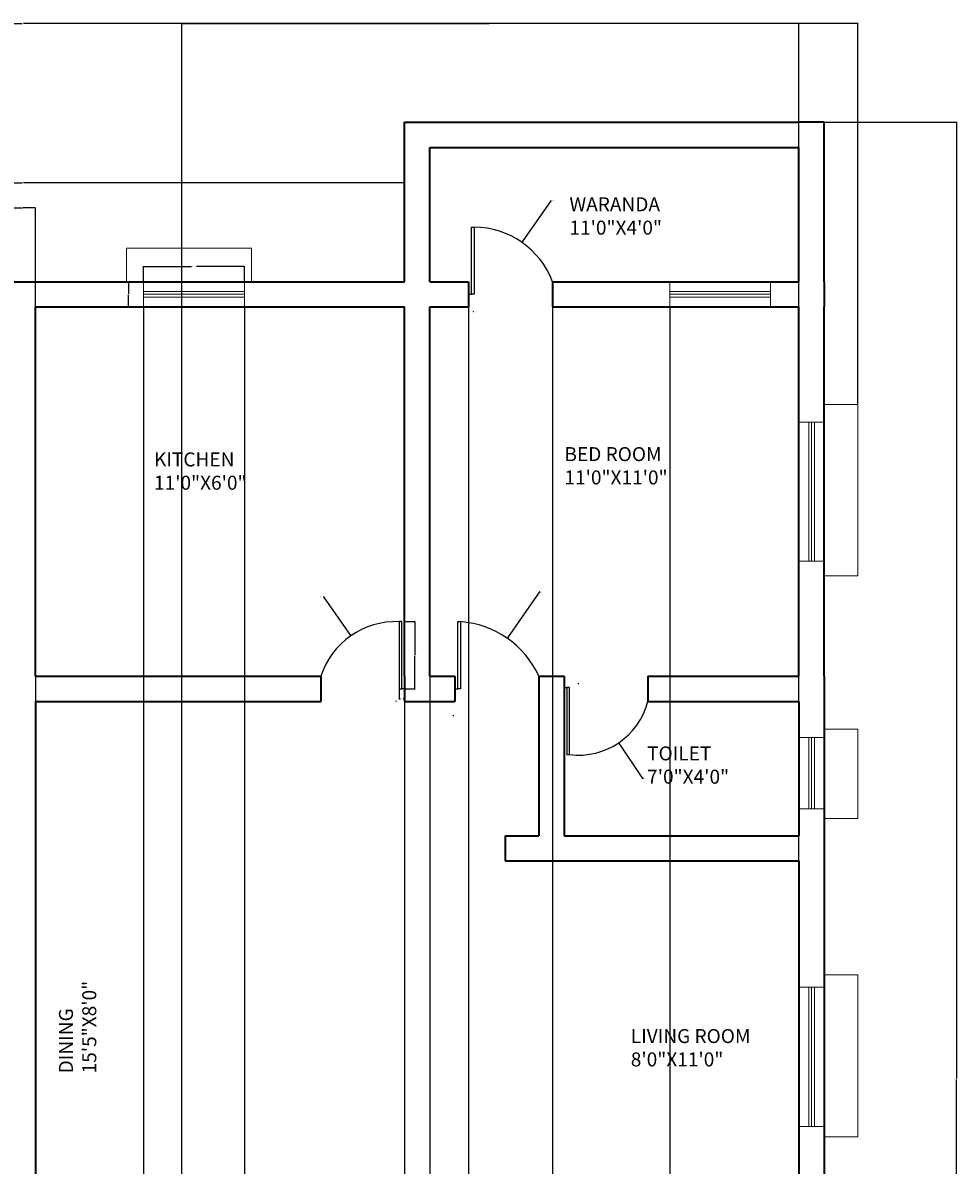
# Model space of a CAD drawing. Units: inches. Extents: x -35 to 633, y -653 to 119.
# Tile 4 of 4: x 299 to 633, y -289 to 119. Entities that reach past the tile are written whole.
import ezdxf

# ---------------------------------------------------------------- set-up
doc = ezdxf.new("R2010")
doc.units = ezdxf.units.IN
doc.header["$MEASUREMENT"] = 0
for name, color, linetype, lineweight in [('A-ANNO-DIMS', 2, 'Continuous', 18), ('A-AREA-IDEN', 7, 'Continuous', 18), ('A-DOOR', 3, 'Continuous', 25), ('A-GLAZ', 4, 'Continuous', 20), ('A-GLAZ-PROJ', 4, 'Continuous', 18), ('A-WALL', 7, 'Continuous', 35)]:
    doc.layers.add(name, color=color, linetype=linetype, lineweight=lineweight)
doc.styles.get("Standard").update_dxf_attribs({"font": 'arial.ttf'})
doc.dimstyles.get("Standard").update_dxf_attribs({"dimtxt": 0.18, "dimasz": 0.18, "dimexe": 0.18, "dimexo": 0.0625, "dimgap": 0.09, "dimtad": 0, "dimtih": 1, "dimtoh": 1, "dimdec": 4, "dimzin": 0, "dimdsep": 46, "dimtxsty": 'Standard', "dimcen": 0.09, "dimadec": 0, "dimazin": 0, "dimtfac": 1, "dimtdec": 4, "dimtofl": 0, "dimtmove": 0, "dimatfit": 3, "dimfxl": 1, "dimtolj": 1, "dimtzin": 0, "dimarcsym": 0})

# ---------------------------------------------------------------- blocks, each defined once
blk = doc.blocks.new('DOOR-LEAF-24IN')
for p, q in [((-1, 24), (-2, 24)), ((-2, 24), (-2, 0)), ((-1, 0), (-1, 24)), ((-2, 0), (-1, 0)), ((0, 0), (-1, 0))]:
    blk.add_line(p, q)
blk = doc.blocks.new('WIN-36IN')
for p, q in [((0, -3.5), (36, -3.5)), ((0, -4.5), (36, -4.5)), ((0, -5.5), (36, -5.5))]:
    blk.add_line(p, q)
blk.add_lwpolyline([(0, 0), (36, 0), (36, -9), (0, -9)], close=True)
blk = doc.blocks.new('*D4')
at = {"layer": 'A-ANNO-DIMS', "color": 0, "lineweight": -2, "transparency": 16777216}
for p, q in [((435.75, -95.21), (439.47, -95.21)), ((439.29, -95.39), (439.29, -107.03)), ((439.29, -119.03), (439.29, -107.39)), ((435.75, -119.21), (439.47, -119.21))]:
    blk.add_line(p, q, dxfattribs=at)
at = {"layer": 'A-ANNO-DIMS', "color": 0, "transparency": 16777216}
for points in [[(439.26, -95.39), (439.32, -95.39), (439.29, -95.21)], [(439.26, -119.03), (439.32, -119.03), (439.29, -119.21)]]:
    blk.add_solid(points, dxfattribs=at)
at = {"layer": 'Defpoints', "color": 0, "transparency": 16777216}
for p in [(435.69, -95.21), (439.29, -95.21), (435.69, -119.21)]:
    blk.add_point(p, dxfattribs=at)
at = {"layer": 'A-ANNO-DIMS', "color": 0, "transparency": 16777216, "insert": (439.29, -107.21), "char_height": 0.18, "attachment_point": 5}
blk.add_mtext('\\A1;LEAF 24 TYP.', dxfattribs=at)
blk = doc.blocks.new('*D5')
at = {"layer": 'A-ANNO-DIMS', "color": 0, "lineweight": -2, "transparency": 16777216}
for p, q in [((433.69, -119.28), (433.69, -122.99)), ((435.69, -119.28), (435.69, -122.99)), ((433.87, -122.81), (434.23, -122.81)), ((435.51, -122.81), (435.15, -122.81))]:
    blk.add_line(p, q, dxfattribs=at)
at = {"layer": 'A-ANNO-DIMS', "color": 0, "transparency": 16777216}
for points in [[(433.87, -122.78), (433.87, -122.84), (433.69, -122.81)], [(435.51, -122.78), (435.51, -122.84), (435.69, -122.81)]]:
    blk.add_solid(points, dxfattribs=at)
at = {"layer": 'Defpoints', "color": 0, "transparency": 16777216}
for p in [(433.69, -119.21), (435.69, -119.21), (435.69, -122.81)]:
    blk.add_point(p, dxfattribs=at)
at = {"layer": 'A-ANNO-DIMS', "color": 0, "transparency": 16777216, "insert": (434.69, -122.81), "char_height": 0.18, "attachment_point": 5}
blk.add_mtext('\\A1;2 TYP.', dxfattribs=at)
blk = doc.blocks.new('*D6')
at = {"layer": 'A-ANNO-DIMS', "color": 0, "lineweight": -2, "transparency": 16777216}
for p, q in [((342.39, 26.35), (342.39, 31.87)), ((342.57, 31.69), (359.54, 31.69)), ((378.21, 31.69), (361.23, 31.69)), ((378.39, 26.35), (378.39, 31.87))]:
    blk.add_line(p, q, dxfattribs=at)
at = {"layer": 'A-ANNO-DIMS', "color": 0, "transparency": 16777216}
for points in [[(342.57, 31.72), (342.57, 31.66), (342.39, 31.69)], [(378.21, 31.72), (378.21, 31.66), (378.39, 31.69)]]:
    blk.add_solid(points, dxfattribs=at)
at = {"layer": 'Defpoints', "color": 0, "transparency": 16777216}
for p in [(378.39, 31.69), (342.39, 26.29), (378.39, 26.29)]:
    blk.add_point(p, dxfattribs=at)
at = {"layer": 'A-ANNO-DIMS', "color": 0, "transparency": 16777216, "insert": (360.39, 31.69), "char_height": 0.18, "attachment_point": 5}
blk.add_mtext('\\A1;WIN. 36 TYP.', dxfattribs=at)
blk = doc.blocks.new('*D7')
at = {"layer": 'A-ANNO-DIMS', "color": 0, "lineweight": -2, "transparency": 16777216}
for p, q in [((342.32, 26.29), (336.81, 26.29)), ((336.99, 26.11), (336.99, 21.97)), ((336.99, 17.47), (336.99, 21.61)), ((342.32, 17.29), (336.81, 17.29))]:
    blk.add_line(p, q, dxfattribs=at)
at = {"layer": 'A-ANNO-DIMS', "color": 0, "transparency": 16777216}
for points in [[(336.96, 26.11), (337.02, 26.11), (336.99, 26.29)], [(336.96, 17.47), (337.02, 17.47), (336.99, 17.29)]]:
    blk.add_solid(points, dxfattribs=at)
at = {"layer": 'Defpoints', "color": 0, "transparency": 16777216}
for p in [(336.99, 26.29), (342.39, 26.29), (342.39, 17.29)]:
    blk.add_point(p, dxfattribs=at)
at = {"layer": 'A-ANNO-DIMS', "color": 0, "transparency": 16777216, "insert": (336.99, 21.79), "char_height": 0.18, "attachment_point": 5}
blk.add_mtext('\\A1;9 TYP.', dxfattribs=at)
blk = doc.blocks.new('*D11')
at = {"layer": 'A-ANNO-DIMS', "color": 0, "lineweight": -2, "transparency": 16777216}
for p, q in [((0.69, -14.75), (0.69, 118.82)), ((0.87, 118.64), (298.9, 118.64)), ((597.51, 118.64), (299.48, 118.64)), ((597.69, -17.48), (597.69, 118.82))]:
    blk.add_line(p, q, dxfattribs=at)
at = {"layer": 'A-ANNO-DIMS', "color": 0, "transparency": 16777216}
for points in [[(0.87, 118.67), (0.87, 118.61), (0.69, 118.64)], [(597.51, 118.67), (597.51, 118.61), (597.69, 118.64)]]:
    blk.add_solid(points, dxfattribs=at)
at = {"layer": 'Defpoints', "color": 0, "transparency": 16777216}
for p in [(597.69, 118.64), (0.69, -14.81), (597.69, -17.55)]:
    blk.add_point(p, dxfattribs=at)
at = {"layer": 'A-ANNO-DIMS', "color": 0, "transparency": 16777216, "insert": (299.19, 118.64), "char_height": 0.18, "attachment_point": 5}
blk.add_mtext('\\A1;597', dxfattribs=at)
blk = doc.blocks.new('*D12')
at = {"layer": 'A-ANNO-DIMS', "color": 0, "lineweight": -2, "transparency": 16777216}
for p, q in [((162.69, 26.35), (162.69, 61.82)), ((162.87, 61.64), (298.9, 61.64)), ((435.51, 61.64), (299.48, 61.64)), ((435.69, 26.35), (435.69, 61.82))]:
    blk.add_line(p, q, dxfattribs=at)
at = {"layer": 'A-ANNO-DIMS', "color": 0, "transparency": 16777216}
for points in [[(162.87, 61.67), (162.87, 61.61), (162.69, 61.64)], [(435.51, 61.67), (435.51, 61.61), (435.69, 61.64)]]:
    blk.add_solid(points, dxfattribs=at)
at = {"layer": 'Defpoints', "color": 0, "transparency": 16777216}
for p in [(435.69, 61.64), (162.69, 26.29), (435.69, 26.29)]:
    blk.add_point(p, dxfattribs=at)
at = {"layer": 'A-ANNO-DIMS', "color": 0, "transparency": 16777216, "insert": (299.19, 61.64), "char_height": 0.18, "attachment_point": 5}
blk.add_mtext('\\A1;273', dxfattribs=at)
blk = doc.blocks.new('*D18')
at = {"layer": 'A-ANNO-DIMS', "color": 0, "lineweight": -2, "transparency": 16777216}
for p, q in [((294.69, 17.35), (294.69, 52.82)), ((294.87, 52.64), (299.04, 52.64)), ((303.51, 52.64), (299.34, 52.64)), ((303.69, 17.35), (303.69, 52.82))]:
    blk.add_line(p, q, dxfattribs=at)
at = {"layer": 'A-ANNO-DIMS', "color": 0, "transparency": 16777216}
for points in [[(294.87, 52.67), (294.87, 52.61), (294.69, 52.64)], [(303.51, 52.67), (303.51, 52.61), (303.69, 52.64)]]:
    blk.add_solid(points, dxfattribs=at)
at = {"layer": 'Defpoints', "color": 0, "transparency": 16777216}
for p in [(303.69, 52.64), (294.69, 17.29), (303.69, 17.29)]:
    blk.add_point(p, dxfattribs=at)
at = {"layer": 'A-ANNO-DIMS', "color": 0, "transparency": 16777216, "insert": (299.19, 52.64), "char_height": 0.18, "attachment_point": 5}
blk.add_mtext('\\A1;9', dxfattribs=at)
blk = doc.blocks.new('*D19')
at = {"layer": 'A-ANNO-DIMS', "color": 0, "lineweight": -2, "transparency": 16777216}
for p, q in [((303.69, 17.22), (303.69, -652.72)), ((342.39, 17.22), (342.39, -652.72)), ((303.87, -652.54), (322.57, -652.54)), ((342.21, -652.54), (323.5, -652.54))]:
    blk.add_line(p, q, dxfattribs=at)
at = {"layer": 'A-ANNO-DIMS', "color": 0, "transparency": 16777216}
for points in [[(303.87, -652.51), (303.87, -652.57), (303.69, -652.54)], [(342.21, -652.51), (342.21, -652.57), (342.39, -652.54)]]:
    blk.add_solid(points, dxfattribs=at)
at = {"layer": 'Defpoints', "color": 0, "transparency": 16777216}
for p in [(303.69, 17.29), (342.39, 17.29), (342.39, -652.54)]:
    blk.add_point(p, dxfattribs=at)
at = {"layer": 'A-ANNO-DIMS', "color": 0, "transparency": 16777216, "insert": (323.04, -652.54), "char_height": 0.18, "attachment_point": 5}
blk.add_mtext('\\A1;38.695', dxfattribs=at)
blk = doc.blocks.new('*D20')
at = {"layer": 'A-ANNO-DIMS', "color": 0, "lineweight": -2, "transparency": 16777216}
for p, q in [((378.39, 17.22), (378.39, -652.72)), ((435.69, 17.22), (435.69, -652.72)), ((378.57, -652.54), (406.71, -652.54)), ((435.51, -652.54), (407.36, -652.54))]:
    blk.add_line(p, q, dxfattribs=at)
at = {"layer": 'A-ANNO-DIMS', "color": 0, "transparency": 16777216}
for points in [[(378.57, -652.51), (378.57, -652.57), (378.39, -652.54)], [(435.51, -652.51), (435.51, -652.57), (435.69, -652.54)]]:
    blk.add_solid(points, dxfattribs=at)
at = {"layer": 'Defpoints', "color": 0, "transparency": 16777216}
for p in [(378.39, 17.29), (435.69, 17.29), (435.69, -652.54)]:
    blk.add_point(p, dxfattribs=at)
at = {"layer": 'A-ANNO-DIMS', "color": 0, "transparency": 16777216, "insert": (407.04, -652.54), "char_height": 0.18, "attachment_point": 5}
blk.add_mtext('\\A1;57.3', dxfattribs=at)
blk = doc.blocks.new('*D21')
at = {"layer": 'A-ANNO-DIMS', "color": 0, "lineweight": -2, "transparency": 16777216}
for p, q in [((444.69, 17.22), (444.69, -652.72)), ((458.58, 17.22), (458.58, -652.72)), ((444.87, -652.54), (451.25, -652.54)), ((458.4, -652.54), (452.02, -652.54))]:
    blk.add_line(p, q, dxfattribs=at)
at = {"layer": 'A-ANNO-DIMS', "color": 0, "transparency": 16777216}
for points in [[(444.87, -652.51), (444.87, -652.57), (444.69, -652.54)], [(458.4, -652.51), (458.4, -652.57), (458.58, -652.54)]]:
    blk.add_solid(points, dxfattribs=at)
at = {"layer": 'Defpoints', "color": 0, "transparency": 16777216}
for p in [(444.69, 17.29), (458.58, 17.29), (458.58, -652.54)]:
    blk.add_point(p, dxfattribs=at)
at = {"layer": 'A-ANNO-DIMS', "color": 0, "transparency": 16777216, "insert": (451.64, -652.54), "char_height": 0.18, "attachment_point": 5}
blk.add_mtext('\\A1;13.89', dxfattribs=at)
blk = doc.blocks.new('*D22')
at = {"layer": 'A-ANNO-DIMS', "color": 0, "lineweight": -2, "transparency": 16777216}
for p, q in [((458.58, 17.22), (458.58, -652.72)), ((488.58, 17.22), (488.58, -652.72)), ((458.76, -652.54), (473.36, -652.54)), ((488.4, -652.54), (473.8, -652.54))]:
    blk.add_line(p, q, dxfattribs=at)
at = {"layer": 'A-ANNO-DIMS', "color": 0, "transparency": 16777216}
for points in [[(458.76, -652.51), (458.76, -652.57), (458.58, -652.54)], [(488.4, -652.51), (488.4, -652.57), (488.58, -652.54)]]:
    blk.add_solid(points, dxfattribs=at)
at = {"layer": 'Defpoints', "color": 0, "transparency": 16777216}
for p in [(458.58, 17.29), (488.58, 17.29), (488.58, -652.54)]:
    blk.add_point(p, dxfattribs=at)
at = {"layer": 'A-ANNO-DIMS', "color": 0, "transparency": 16777216, "insert": (473.58, -652.54), "char_height": 0.18, "attachment_point": 5}
blk.add_mtext('\\A1;30', dxfattribs=at)
blk = doc.blocks.new('*D23')
at = {"layer": 'A-ANNO-DIMS', "color": 0, "lineweight": -2, "transparency": 16777216}
for p, q in [((488.58, 17.22), (488.58, -652.72)), ((530.49, 17.22), (530.49, -652.72)), ((488.76, -652.54), (509.15, -652.54)), ((530.31, -652.54), (509.91, -652.54))]:
    blk.add_line(p, q, dxfattribs=at)
at = {"layer": 'A-ANNO-DIMS', "color": 0, "transparency": 16777216}
for points in [[(488.76, -652.51), (488.76, -652.57), (488.58, -652.54)], [(530.31, -652.51), (530.31, -652.57), (530.49, -652.54)]]:
    blk.add_solid(points, dxfattribs=at)
at = {"layer": 'Defpoints', "color": 0, "transparency": 16777216}
for p in [(488.58, 17.29), (530.49, 17.29), (530.49, -652.54)]:
    blk.add_point(p, dxfattribs=at)
at = {"layer": 'A-ANNO-DIMS', "color": 0, "transparency": 16777216, "insert": (509.53, -652.54), "char_height": 0.18, "attachment_point": 5}
blk.add_mtext('\\A1;41.91', dxfattribs=at)
blk = doc.blocks.new('*D24')
at = {"layer": 'A-ANNO-DIMS', "color": 0, "lineweight": -2, "transparency": 16777216}
for p, q in [((585.75, 83.29), (633.22, 83.29)), ((633.04, 83.11), (633.04, -258.53)), ((633.04, -600.53), (633.04, -258.89)), ((356.04, -600.71), (633.22, -600.71))]:
    blk.add_line(p, q, dxfattribs=at)
at = {"layer": 'A-ANNO-DIMS', "color": 0, "transparency": 16777216}
for points in [[(633.01, 83.11), (633.07, 83.11), (633.04, 83.29)], [(633.01, -600.53), (633.07, -600.53), (633.04, -600.71)]]:
    blk.add_solid(points, dxfattribs=at)
at = {"layer": 'Defpoints', "color": 0, "transparency": 16777216}
for p in [(585.69, 83.29), (355.98, -600.71), (633.04, -600.71)]:
    blk.add_point(p, dxfattribs=at)
at = {"layer": 'A-ANNO-DIMS', "color": 0, "transparency": 16777216, "insert": (633.04, -258.71), "char_height": 0.18, "attachment_point": 5}
blk.add_mtext('\\A1;684', dxfattribs=at)
blk = doc.blocks.new('*D37')
at = {"layer": 'A-ANNO-DIMS', "color": 0, "lineweight": -2, "transparency": 16777216}
for p, q in [((355.98, -546.65), (355.98, 118.82)), ((356.16, 118.64), (465.94, 118.64)), ((576.51, 118.64), (466.73, 118.64)), ((576.69, -546.65), (576.69, 118.82))]:
    blk.add_line(p, q, dxfattribs=at)
at = {"layer": 'A-ANNO-DIMS', "color": 0, "transparency": 16777216}
for points in [[(356.16, 118.67), (356.16, 118.61), (355.98, 118.64)], [(576.51, 118.67), (576.51, 118.61), (576.69, 118.64)]]:
    blk.add_solid(points, dxfattribs=at)
at = {"layer": 'Defpoints', "color": 0, "transparency": 16777216}
for p in [(576.69, 118.64), (355.98, -546.71), (576.69, -546.71)]:
    blk.add_point(p, dxfattribs=at)
at = {"layer": 'A-ANNO-DIMS', "color": 0, "transparency": 16777216, "insert": (466.33, 118.64), "char_height": 0.18, "attachment_point": 5}
blk.add_mtext('\\A1;220.7', dxfattribs=at)
blk = doc.blocks.new('*D48')
at = {"layer": 'A-ANNO-DIMS', "color": 0, "lineweight": -2, "transparency": 16777216}
for p, q in [((303.69, -123.78), (303.69, -652.72)), ((483.69, -312.78), (483.69, -652.72)), ((303.87, -652.54), (393.41, -652.54)), ((483.51, -652.54), (393.97, -652.54))]:
    blk.add_line(p, q, dxfattribs=at)
at = {"layer": 'A-ANNO-DIMS', "color": 0, "transparency": 16777216}
for points in [[(303.87, -652.51), (303.87, -652.57), (303.69, -652.54)], [(483.51, -652.51), (483.51, -652.57), (483.69, -652.54)]]:
    blk.add_solid(points, dxfattribs=at)
at = {"layer": 'Defpoints', "color": 0, "transparency": 16777216}
for p in [(303.69, -123.71), (483.69, -312.71), (483.69, -652.54)]:
    blk.add_point(p, dxfattribs=at)
at = {"layer": 'A-ANNO-DIMS', "color": 0, "transparency": 16777216, "insert": (393.69, -652.54), "char_height": 0.18, "attachment_point": 5}
blk.add_mtext('\\A1;180', dxfattribs=at)
blk = doc.blocks.new('*D50')
at = {"layer": 'A-ANNO-DIMS', "color": 0, "lineweight": -2, "transparency": 16777216}
for p, q in [((483.87, -84.6), (472.45, -101)), ((484.05, -84.6), (483.87, -84.6)), ((453.05, -128.73), (453.23, -128.73)), ((453.14, -128.82), (453.14, -128.64))]:
    blk.add_line(p, q, dxfattribs=at)
at = {"layer": 'A-ANNO-DIMS', "color": 0, "transparency": 16777216}
blk.add_solid([(472.43, -100.98), (472.48, -101.01), (472.35, -101.15)], dxfattribs=at)
at = {"layer": 'Defpoints', "color": 0, "transparency": 16777216}
for p in [(472.35, -101.15), (453.14, -128.73)]:
    blk.add_point(p, dxfattribs=at)
at = {"layer": 'A-ANNO-DIMS', "color": 0, "transparency": 16777216, "insert": (484.52, -84.6), "char_height": 0.18, "attachment_point": 5}
blk.add_mtext('\\A1;R33.61', dxfattribs=at)
blk = doc.blocks.new('*D51')
at = {"layer": 'A-ANNO-DIMS', "color": 0, "lineweight": -2, "transparency": 16777216}
for p, q in [((487.95, 55.23), (477.7, 40.52)), ((488.13, 55.23), (487.95, 55.23)), ((460.26, 15.61), (460.44, 15.61)), ((460.35, 15.52), (460.35, 15.7))]:
    blk.add_line(p, q, dxfattribs=at)
at = {"layer": 'A-ANNO-DIMS', "color": 0, "transparency": 16777216}
blk.add_solid([(477.68, 40.54), (477.73, 40.5), (477.6, 40.37)], dxfattribs=at)
at = {"layer": 'Defpoints', "color": 0, "transparency": 16777216}
for p in [(477.6, 40.37), (460.35, 15.61)]:
    blk.add_point(p, dxfattribs=at)
at = {"layer": 'A-ANNO-DIMS', "color": 0, "transparency": 16777216, "insert": (488.61, 55.23), "char_height": 0.18, "attachment_point": 5}
blk.add_mtext('\\A1;R30.18', dxfattribs=at)
blk = doc.blocks.new('*D53')
at = {"layer": 'A-ANNO-DIMS', "color": 0, "lineweight": -2, "transparency": 16777216}
for p, q in [((406.52, -86.31), (406.7, -86.31)), ((406.7, -86.31), (416.33, -100.14)), ((432.56, -123.58), (432.74, -123.58)), ((432.65, -123.67), (432.65, -123.49))]:
    blk.add_line(p, q, dxfattribs=at)
at = {"layer": 'A-ANNO-DIMS', "color": 0, "transparency": 16777216}
blk.add_solid([(416.35, -100.12), (416.31, -100.16), (416.43, -100.29)], dxfattribs=at)
at = {"layer": 'Defpoints', "color": 0, "transparency": 16777216}
for p in [(416.43, -100.29), (432.65, -123.58)]:
    blk.add_point(p, dxfattribs=at)
at = {"layer": 'A-ANNO-DIMS', "color": 0, "transparency": 16777216, "insert": (405.97, -86.31), "char_height": 0.18, "attachment_point": 5}
blk.add_mtext('\\A1;R28.383', dxfattribs=at)
blk = doc.blocks.new('*D58')
at = {"layer": 'A-ANNO-DIMS', "color": 0, "lineweight": -2, "transparency": 16777216}
for p, q in [((497.79, -117.29), (497.97, -117.29)), ((497.88, -117.38), (497.88, -117.2)), ((520.91, -151.22), (512.38, -138.64)), ((521.09, -151.22), (520.91, -151.22))]:
    blk.add_line(p, q, dxfattribs=at)
at = {"layer": 'A-ANNO-DIMS', "color": 0, "transparency": 16777216}
blk.add_solid([(512.4, -138.63), (512.35, -138.66), (512.27, -138.49)], dxfattribs=at)
at = {"layer": 'Defpoints', "color": 0, "transparency": 16777216}
for p in [(497.88, -117.29), (512.27, -138.49)]:
    blk.add_point(p, dxfattribs=at)
at = {"layer": 'A-ANNO-DIMS', "color": 0, "transparency": 16777216, "insert": (521.57, -151.22), "char_height": 0.18, "attachment_point": 5}
blk.add_mtext('\\A1;R25.63', dxfattribs=at)

msp = doc.modelspace()

# ---------------------------------------------------------------- linework, layer by layer
at = {"layer": 'A-DOOR'}
for centre, radius, start, end in [((460.3538, 15.6104), 30.1775, 20.719567, 89.571521), ((432.654, -123.577), 28.3829, 87.90681, 161.802101), ((453.1421, -128.7251), 33.6089, 24.64007, 85.651018), ((497.8804, -117.2907), 25.628, 262.850149, 345.487272)]:
    msp.add_arc(centre, radius, start, end, dxfattribs=at)
at = {"layer": 'A-GLAZ'}
for p, q in [((576.6907, -23.96), (585.6907, -23.96)), ((580.1907, -23.96), (580.1907, -73.5465)), ((581.1907, -23.96), (581.1907, -73.5465)), ((582.1907, -23.96), (582.1907, -73.5465)), ((576.6907, -73.5465), (585.6907, -73.5465)), ((576.6907, -136.6242), (585.6907, -136.6242)), ((580.1907, -136.6242), (580.1907, -162.1051)), ((581.1907, -136.6242), (581.1907, -162.1051)), ((582.1907, -136.6242), (582.1907, -162.1051)), ((576.6907, -162.1051), (585.6907, -162.1051)), ((576.6907, -225.9037), (585.6907, -225.9037)), ((580.1907, -225.9037), (580.1907, -275.7093)), ((581.1907, -225.9037), (581.1907, -275.7093)), ((582.1907, -225.9037), (582.1907, -275.7093)), ((576.6907, -275.7093), (585.6907, -275.7093))]:
    msp.add_line(p, q, dxfattribs=at)
at = {"layer": 'A-GLAZ-PROJ'}
for p, q in [((336.219, 26.287), (336.219, 38.287)), ((336.219, 38.287), (380.9785, 38.287)), ((380.9785, 38.287), (380.9785, 26.287)), ((585.6907, -17.5469), (597.6907, -17.5469)), ((597.6907, -17.5469), (597.6907, -78.8543)), ((597.6907, -78.8543), (585.6907, -78.8543)), ((585.6907, -133.5845), (597.6907, -133.5845)), ((597.6907, -133.5845), (597.6907, -165.5926)), ((597.6907, -165.5926), (585.6907, -165.5926)), ((585.6907, -221.426), (597.6907, -221.426)), ((597.6907, -221.426), (597.6907, -279.3152)), ((597.6907, -279.3152), (585.6907, -279.3152))]:
    msp.add_line(p, q, dxfattribs=at)
at = {"layer": 'A-WALL'}
for p, q in [((435.6907, 26.287), (435.6907, 83.287)), ((435.6907, 83.287), (576.6907, 83.287)), ((585.6907, 83.287), (576.6907, 83.287)), ((585.6907, 26.287), (585.6907, 83.287)), ((444.6907, 26.287), (444.6907, 74.287)), ((444.6907, 74.287), (576.6907, 74.287)), ((576.6907, 26.287), (576.6907, 74.287)), ((162.6907, 26.287), (435.6907, 26.287)), ((444.6907, 26.287), (458.5795, 26.287)), ((458.5795, 26.287), (458.5795, 17.287)), ((488.5795, 26.287), (488.5795, 17.287)), ((488.5795, 26.287), (576.6907, 26.287)), ((585.6907, 26.287), (585.6907, 17.287)), ((303.6907, -114.713), (303.6907, 17.287)), ((303.6907, 17.287), (435.6907, 17.287)), ((435.6907, -114.713), (435.6907, 17.287)), ((444.6907, -114.713), (444.6907, 17.287)), ((444.6907, 17.287), (458.5795, 17.287)), ((488.5795, 17.287), (576.6907, 17.287)), ((576.6907, -114.713), (576.6907, 17.287)), ((585.6907, -114.713), (585.6907, 17.287)), ((303.6907, -114.713), (405.6907, -114.713)), ((405.6907, -114.713), (405.6907, -123.713)), ((435.6907, -114.713), (435.6907, -123.713)), ((444.6907, -114.713), (453.6907, -114.713)), ((453.6907, -114.713), (453.6907, -123.713)), ((483.6907, -114.713), (483.6907, -171.713)), ((483.6907, -114.713), (492.6907, -114.713)), ((492.6907, -114.713), (492.6907, -171.713)), ((522.6907, -114.713), (522.6907, -123.713)), ((522.6907, -114.713), (576.6907, -114.713)), ((585.6907, -114.713), (585.6907, -555.713)), ((303.6907, -123.713), (303.6907, -389.6034)), ((303.6907, -123.713), (405.6907, -123.713)), ((435.6907, -123.713), (453.6907, -123.713)), ((522.6907, -123.713), (576.6907, -123.713)), ((576.6907, -123.713), (576.6907, -171.713)), ((471.6907, -171.713), (483.6907, -171.713)), ((471.6907, -171.713), (471.6907, -180.713)), ((492.6907, -171.713), (576.6907, -171.713)), ((471.6907, -180.713), (483.2432, -180.713)), ((480.6907, -180.713), (576.6907, -180.713)), ((576.6907, -180.713), (576.6907, -312.713))]:
    msp.add_line(p, q, dxfattribs=at)

# ---------------------------------------------------------------- block references
at = {"layer": 'A-DOOR', "extrusion": (0, 0, -1), "zscale": -1}
for p in [(-458.5795, 21.787), (-453.6907, -119.213)]:
    msp.add_blockref('DOOR-LEAF-24IN', p, dxfattribs=at)
at = {"layer": 'A-DOOR'}
msp.add_blockref('DOOR-LEAF-24IN', (435.6907, -119.213), dxfattribs=at)
at = {"layer": 'A-DOOR', "rotation": 180}
msp.add_blockref('DOOR-LEAF-24IN', (492.6907, -118.7194), dxfattribs=at)
at = {"layer": 'A-GLAZ'}
for p in [(342.3856, 26.287), (530.4897, 26.287)]:
    msp.add_blockref('WIN-36IN', p, dxfattribs=at)

# ---------------------------------------------------------------- texts
at = {"layer": 'A-AREA-IDEN', "char_height": 5, "attachment_point": 1}
for s, width, insert in [('WARANDA\\P11\'0"X4\'0"', 24.624866, (494.6203, 56.4574)), ('KITCHEN\\P11\'0"X6\'0"', 40.946262, (346.0831, -34.7212)), ('BED ROOM\\P11\'0"X11\'0"', 64.884056, (492.8345, -32.8336)), ('TOILET\\P7\'0"X4\'0"', 26.587234, (522.3969, -139.7929)), ('LIVING ROOM\\P8\'0"X11\'0"', 66.509643, (516.5563, -240.8356))]:
    msp.add_mtext_dynamic_manual_height_columns(s, width=width, gutter_width=25, heights=[0], dxfattribs=dict(at, insert=insert))
at = {"layer": 'A-AREA-IDEN', "insert": (312.1128, -256.6764), "char_height": 5, "attachment_point": 1, "rotation": 90}
msp.add_mtext_dynamic_manual_height_columns('DINING\\P15\'5"X8\'0"', width=68.431972, gutter_width=25, heights=[0], dxfattribs=at)

# ---------------------------------------------------------------- dimensions: what is measured, and where the dimension line sits
at = {"layer": 'A-ANNO-DIMS'}
for base, p1, p2, override, picture, middle in [((597.6907, 118.637), (0.6907, -14.8086), (597.6907, -17.5469), {"dimdec": 0, "dimlfac": 1, "dimrnd": 0, "dimzin": 0, "dimdsep": 46, "dimlunit": 2}, '*D11', (299.1907, 118.637)), ((576.6907, 118.637), (355.9768, -546.713), (576.6907, -546.713), {"dimdec": 1, "dimlfac": 1, "dimrnd": 0, "dimzin": 0, "dimdsep": 46, "dimlunit": 2}, '*D37', (466.3337, 118.637)), ((435.6907, 61.637), (162.6907, 26.287), (435.6907, 26.287), {"dimdec": 0, "dimlfac": 1, "dimrnd": 0, "dimzin": 0, "dimdsep": 46, "dimlunit": 2}, '*D12', (299.1907, 61.637)), ((303.6907, 52.637), (294.6907, 17.287), (303.6907, 17.287), {"dimdec": 0, "dimlfac": 1, "dimrnd": 0, "dimzin": 0, "dimdsep": 46, "dimlunit": 2}, '*D18', (299.1907, 52.637)), ((342.3856, -652.537), (303.6907, 17.287), (342.3856, 17.287), {"dimdec": 3, "dimlfac": 1, "dimrnd": 0, "dimzin": 0, "dimdsep": 46, "dimlunit": 2}, '*D19', (323.0381, -652.537)), ((435.6907, -652.537), (378.3856, 17.287), (435.6907, 17.287), {"dimdec": 1, "dimlfac": 1, "dimrnd": 0, "dimzin": 0, "dimdsep": 46, "dimlunit": 2}, '*D20', (407.0381, -652.537)), ((458.5795, -652.537), (444.6907, 17.287), (458.5795, 17.287), {"dimdec": 2, "dimlfac": 1, "dimrnd": 0, "dimzin": 0, "dimdsep": 46, "dimlunit": 2}, '*D21', (451.6351, -652.537)), ((488.5795, -652.537), (458.5795, 17.287), (488.5795, 17.287), {"dimdec": 0, "dimlfac": 1, "dimrnd": 0, "dimzin": 0, "dimdsep": 46, "dimlunit": 2}, '*D22', (473.5795, -652.537)), ((530.4897, -652.537), (488.5795, 17.287), (530.4897, 17.287), {"dimdec": 2, "dimlfac": 1, "dimrnd": 0, "dimzin": 0, "dimdsep": 46, "dimlunit": 2}, '*D23', (509.5346, -652.537)), ((483.6907, -652.537), (303.6907, -123.713), (483.6907, -312.713), {"dimdec": 0, "dimlfac": 1, "dimrnd": 0, "dimzin": 0, "dimdsep": 46, "dimlunit": 2}, '*D48', (393.6907, -652.537))]:
    dim = msp.add_linear_dim(base=base, p1=p1, p2=p2, dimstyle='Standard', override=override, dxfattribs=at)
    dim.commit()
    dim.dimension.update_dxf_attribs({"geometry": picture, "text_midpoint": middle})
dim = msp.add_linear_dim(base=(633.0407, -600.713), p1=(585.6907, 83.287), p2=(355.9768, -600.713), angle=90, dimstyle='Standard', override={"dimdec": 0, "dimlfac": 1, "dimrnd": 0, "dimzin": 0, "dimdsep": 46, "dimlunit": 2}, dxfattribs=at)
dim.commit()
dim.dimension.update_dxf_attribs({"geometry": '*D24', "text_midpoint": (633.0407, -258.713)})
for center, mpoint, override, picture, middle in [((460.3538, 15.6104), (477.6001, 40.3742), {"dimdec": 2, "dimlfac": 1, "dimrnd": 0, "dimzin": 0, "dimdsep": 46, "dimlunit": 2}, '*D51', (488.6079, 55.2324)), ((453.1421, -128.7251), (472.3489, -101.1451), {"dimdec": 2, "dimlfac": 1, "dimrnd": 0, "dimzin": 0, "dimdsep": 46, "dimlunit": 2}, '*D50', (484.5155, -84.5972)), ((432.654, -123.577), (416.433, -100.286), {"dimdec": 3, "dimlfac": 1, "dimrnd": 0, "dimzin": 0, "dimdsep": 46, "dimlunit": 2}, '*D53', (405.9706, -86.3114)), ((497.8804, -117.2907), (512.274, -138.4949), {"dimdec": 2, "dimlfac": 1, "dimrnd": 0, "dimzin": 0, "dimdsep": 46, "dimlunit": 2}, '*D58', (521.5699, -151.2175))]:
    dim = msp.add_radius_dim(center=center, mpoint=mpoint, dimstyle='Standard', override=override, dxfattribs=at)
    dim.commit()
    dim.dimension.update_dxf_attribs({"geometry": picture, "text_midpoint": middle, "dimtype": 164})
for base, p1, p2, text, picture, middle in [((378.3856, 31.687), (342.3856, 26.287), (378.3856, 26.287), 'WIN. <> TYP.', '*D6', (360.3856, 31.687)), ((435.6907, -122.813), (433.6907, -119.213), (435.6907, -119.213), '<> TYP.', '*D5', (434.6907, -122.813))]:
    dim = msp.add_linear_dim(base=base, p1=p1, p2=p2, text=text, dimstyle='Standard', override={"dimdec": 0, "dimlfac": 1, "dimrnd": 0, "dimzin": 0, "dimdsep": 46, "dimlunit": 2}, dxfattribs=at)
    dim.commit()
    dim.dimension.update_dxf_attribs({"geometry": picture, "text_midpoint": middle})
for base, p1, p2, text, picture, middle in [((336.9856, 26.287), (342.3856, 17.287), (342.3856, 26.287), '<> TYP.', '*D7', (336.9856, 21.787)), ((439.2907, -95.213), (435.6907, -119.213), (435.6907, -95.213), 'LEAF <> TYP.', '*D4', (439.2907, -107.213))]:
    dim = msp.add_linear_dim(base=base, p1=p1, p2=p2, angle=90, text=text, dimstyle='Standard', override={"dimdec": 0, "dimlfac": 1, "dimrnd": 0, "dimzin": 0, "dimdsep": 46, "dimlunit": 2}, dxfattribs=at)
    dim.commit()
    dim.dimension.update_dxf_attribs({"geometry": picture, "text_midpoint": middle})

doc.saveas('drawing.dxf')
